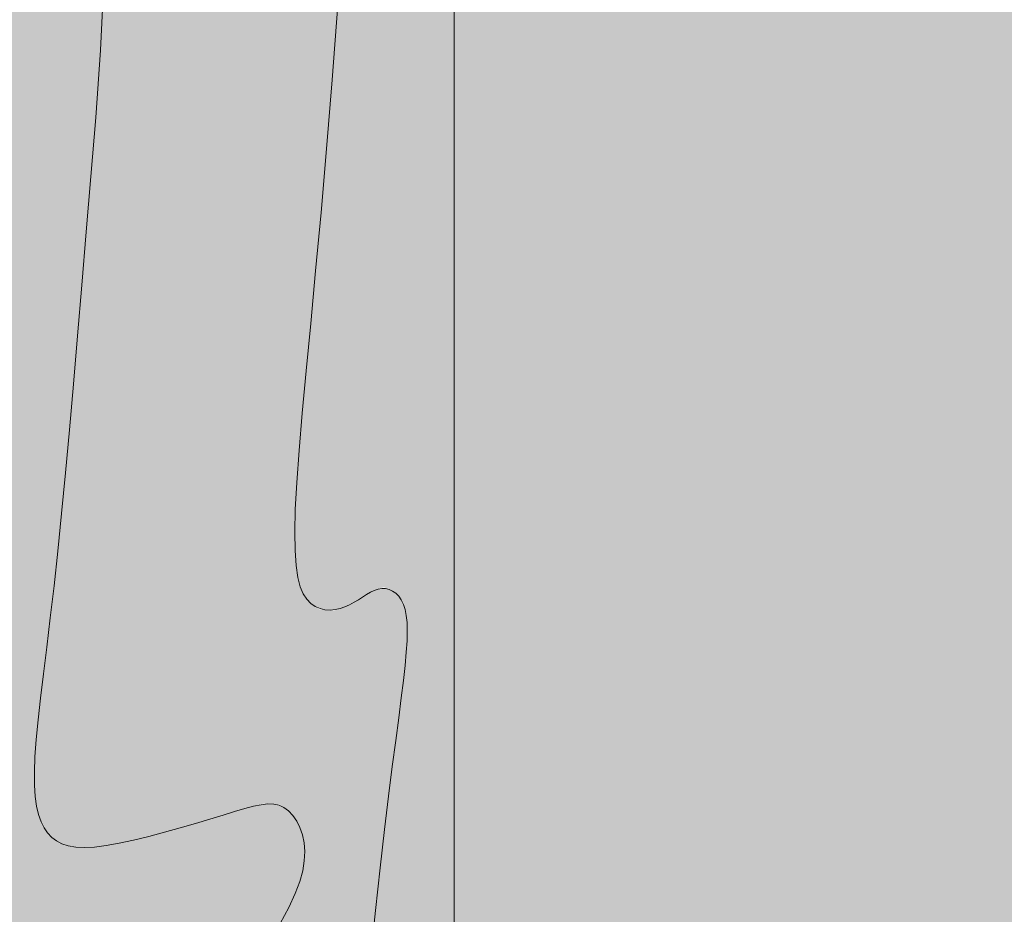
# Model space of a CAD drawing. Units: inches. Extents: x 3024 to 3952, y 1308 to 1863.
# Tile 17 of 29: x 3411.08 to 3430.42, y 1506.34 to 1523.92. Entities that reach past the tile are written whole.
import ezdxf

# ---------------------------------------------------------------- set-up
doc = ezdxf.new("R2010")
doc.units = ezdxf.units.IN
for name, color, linetype, lineweight in [('A-ANNO-DIMS', 2, 'Continuous', 18), ('A-FLOR-TILE-PATT', 7, 'Continuous', 13), ('A-FURN', 8, 'Continuous', 18), ('A-FURN-PATT', 9, 'Continuous', 13)]:
    doc.layers.add(name, color=color, linetype=linetype, lineweight=lineweight)
doc.layers.add('A-FLOR-PATT', color=254, linetype='Continuous', lineweight=13, true_color=0xfeeab9)
doc.styles.get("Standard").update_dxf_attribs({"font": 'arial.ttf'})
doc.dimstyles.get("Standard").update_dxf_attribs({"dimtxt": 0.18, "dimasz": 0.18, "dimexe": 0.18, "dimexo": 0.0625, "dimgap": 0.09, "dimtad": 0, "dimtih": 1, "dimtoh": 1, "dimdec": 4, "dimzin": 0, "dimdsep": 46, "dimtxsty": 'Standard', "dimcen": 0.09, "dimadec": 0, "dimazin": 0, "dimtfac": 1, "dimtdec": 4, "dimtofl": 0, "dimtmove": 0, "dimatfit": 3, "dimfxl": 1, "dimtolj": 1, "dimtzin": 0, "dimarcsym": 0})

# ---------------------------------------------------------------- blocks, each defined once
blk = doc.blocks.new('Table - Rectangular Woodgrain 60 x 30 in.')
blk.add_line((60, 0), (0, 0))
for points in [[(23.3616, -3.0508), (25.3333, -3.2), (27.1477, -3.3495), (28.8172, -3.4958), (30.3437, -3.636), (31.7291, -3.7667), (32.9756, -3.8849), (34.0849, -3.9875), (35.059, -4.0714), (35.9, -4.1334), (36.6114, -4.1711), (37.2041, -4.1854), (37.6906, -4.1779), (38.0833, -4.15), (38.3948, -4.1034), (38.6375, -4.0396), (38.8239, -3.9602), (38.9666, -3.8667), (39.0764, -3.7608), (39.1573, -3.6448), (39.2116, -3.521), (39.2416, -3.3917), (39.2498, -3.2593), (39.2385, -3.1261), (39.21, -2.9944), (39.1666, -2.8667), (39.111, -2.7447), (39.0468, -2.6281), (38.978, -2.5163), (38.9083, -2.4083), (38.8418, -2.3035), (38.7823, -2.201), (38.7337, -2.1001), (38.7, -2), (38.6844, -1.9003), (38.6875, -1.8021), (38.7094, -1.707), (38.75, -1.6167), (38.8094, -1.5326), (38.8875, -1.4563), (38.9844, -1.3893), (39.1, -1.3333), (39.2351, -1.2896), (39.3937, -1.2583), (39.5804, -1.2396), (39.8, -1.2333), (40.057, -1.2396), (40.3562, -1.2583), (40.7023, -1.2896), (41.1, -1.3333), (41.5547, -1.3895), (42.0755, -1.4573), (42.6721, -1.5361), (43.3542, -1.625), (44.1316, -1.7233), (45.014, -1.8302), (46.0114, -1.9449), (47.1333, -2.0667), (48.3862, -2.1947)], [(22.3952, -9.1759), (24.5531, -9.2844), (26.322, -9.4069), (27.8666, -9.5333), (29.3241, -9.6553), (30.7203, -9.7719), (32.0532, -9.8837), (33.3208, -9.9917), (34.5213, -10.0965), (35.6526, -10.199), (36.7128, -10.2999), (37.7, -10.4), (38.6129, -10.4996), (39.4531, -10.5969), (40.223, -10.6895), (40.925, -10.775), (41.5613, -10.8512), (42.1344, -10.9156), (42.6465, -10.966), (43.1, -11), (43.4976, -11.0158), (43.8437, -11.0136), (44.143, -10.9942), (44.4, -10.9583), (44.6195, -10.9069), (44.8062, -10.8406), (44.9648, -10.7603), (45.1, -10.6667), (45.2155, -10.5598), (45.3114, -10.4365), (45.3871, -10.2929), (45.4416, -10.125), (45.4743, -9.929), (45.4844, -9.7011), (45.4709, -9.4371), (45.4333, -9.1333), (45.3716, -8.7883), (45.2896, -8.4104), (45.1919, -8.0107), (45.0833, -7.6), (44.9685, -7.1893), (44.8521, -6.7896), (44.7388, -6.4117), (44.6333, -6.0667), (44.54, -5.7628), (44.4614, -5.4979), (44.4001, -5.2675), (44.3583, -5.0667), (44.3384, -4.8909), (44.3427, -4.7354), (44.3736, -4.5956), (44.4333, -4.4667), (44.5236, -4.3453), (44.6427, -4.2333), (44.7884, -4.1339), (44.9583, -4.05), (45.1501, -3.9849), (45.3614, -3.9417), (45.59, -3.9234), (45.8333, -3.9333), (46.0915, -3.9749), (46.3734, -4.0531), (46.6906, -4.1736), (47.0542, -4.3417), (47.4756, -4.5629)]]:
    blk.add_lwpolyline(points)
blk = doc.blocks.new('*D104')
at = {"layer": 'A-ANNO-DIMS', "color": 0, "lineweight": -2, "transparency": 16777216}
for p, q in [((3360.738, 1515.697), (3360.738, 1515.877)), ((3360.648, 1515.787), (3360.828, 1515.787)), ((3507.355, 1515.787), (3452.554, 1515.787))]:
    blk.add_line(p, q, dxfattribs=at)
at = {"layer": 'A-ANNO-DIMS', "color": 0, "transparency": 16777216}
blk.add_solid([(3452.554, 1515.817), (3452.554, 1515.757), (3452.374, 1515.787)], dxfattribs=at)
at = {"layer": 'Defpoints', "color": 0, "transparency": 16777216}
for p in [(3360.738, 1515.787), (3452.374, 1515.787)]:
    blk.add_point(p, dxfattribs=at)
at = {"layer": 'A-ANNO-DIMS', "color": 0, "transparency": 16777216, "insert": (3507.835, 1515.787), "char_height": 0.18, "attachment_point": 5}
blk.add_mtext('\\A1;R91.64', dxfattribs=at)
blk = doc.blocks.new('*D105')
at = {"layer": 'A-ANNO-DIMS', "color": 0, "lineweight": -2, "transparency": 16777216}
for p, q in [((3370.527, 1515.697), (3370.527, 1515.877)), ((3370.437, 1515.787), (3370.617, 1515.787)), ((3508.74, 1515.787), (3457.09, 1515.787))]:
    blk.add_line(p, q, dxfattribs=at)
at = {"layer": 'A-ANNO-DIMS', "color": 0, "transparency": 16777216}
blk.add_solid([(3457.09, 1515.817), (3457.09, 1515.757), (3456.91, 1515.787)], dxfattribs=at)
at = {"layer": 'Defpoints', "color": 0, "transparency": 16777216}
for p in [(3370.527, 1515.787), (3456.91, 1515.787)]:
    blk.add_point(p, dxfattribs=at)
at = {"layer": 'A-ANNO-DIMS', "color": 0, "transparency": 16777216, "insert": (3509.22, 1515.787), "char_height": 0.18, "attachment_point": 5}
blk.add_mtext('\\A1;R86.38', dxfattribs=at)

msp = doc.modelspace()

# ---------------------------------------------------------------- hatches: boundary and pattern name
at = {"layer": 'A-FLOR-PATT', "transparency": 33554528}
h = msp.add_hatch(color=256, dxfattribs=at)
h.dxf.hatch_style = 1
h.paths.add_polyline_path([(3460.764, 1688.6064), (3412.764, 1688.6064), (3412.764, 1694.6064), (3460.764, 1694.6064), (3460.764, 1778.6064), (3406.764, 1778.6064), (3406.764, 1759.9514), (3318.2981, 1759.9514), (3318.2981, 1658.6064), (3322.5356, 1658.6064), (3322.5356, 1652.6064), (3292.764, 1652.6064), (3292.764, 1778.6064), (3106.764, 1778.6064), (3106.764, 1628.6064), (3172.764, 1628.6064), (3172.764, 1532.6064), (3166.764, 1532.6064), (3166.764, 1628.6064), (3106.764, 1628.6064), (3106.764, 1356.8452), (3202.812, 1356.8452), (3202.812, 1354.2534), (3202.812, 1353.8388), (3202.812, 1351.1212), (3202.812, 1347.8452), (3277.764, 1347.8452), (3277.764, 1353.8452), (3277.764, 1356.8452), (3277.764, 1442.6064), (3460.764, 1442.6064)])
h.paths.add_polyline_path([(3216.238, 1527.2064), (3216.238, 1491.2064), (3214.663, 1491.2064), (3214.663, 1491.2409, -0.3966224), (3180.243, 1526.6064), (3163.0285, 1526.6064), (3163.0285, 1531.1064), (3161.716, 1531.1064), (3161.716, 1561.1064), (3163.0285, 1561.1064), (3163.0285, 1531.1064), (3163.0285, 1526.6064), (3180.243, 1526.6064, 0.3966224), (3214.663, 1491.2409), (3214.663, 1527.2064)], flags=16)
h.paths.add_polyline_path([(3227.364, 1649.8972), (3191.364, 1649.8972), (3191.364, 1651.4722), (3227.364, 1651.4722)], flags=16)
h.paths.add_polyline_path([(3323.1172, 1606.7362), (3323.8545, 1606.8514), (3323.8545, 1594.8241), (3323.1172, 1594.9393)], flags=16)
h.paths.add_polyline_path([(3324.2232, 1606.909), (3330.1216, 1607.8307), (3330.1216, 1614.1093), (3339.3495, 1614.1093), (3340.2711, 1620.0078), (3352.4136, 1620.0078), (3353.3353, 1614.1093), (3359.9941, 1614.1093), (3360.9157, 1620.0078), (3373.0582, 1620.0078), (3373.9799, 1614.1093), (3383.2077, 1614.1093), (3383.2077, 1607.8307), (3389.1062, 1606.909), (3389.1062, 1594.7665), (3383.2077, 1593.8449), (3383.2077, 1587.5663), (3373.9799, 1587.5663), (3373.0583, 1581.6678), (3360.9157, 1581.6678), (3359.9941, 1587.5663), (3353.3353, 1587.5663), (3352.4136, 1581.6678), (3340.2711, 1581.6678), (3339.3495, 1587.5663), (3330.1216, 1587.5663), (3330.1216, 1593.8449), (3324.2232, 1594.7665)], flags=16)
h.paths.add_polyline_path([(3236.1584, 1693.1064), (3236.1584, 1723.1064), (3237.4709, 1723.1064), (3237.4709, 1693.1064)], flags=16)
h.paths.add_polyline_path([(3373.2158, 1600.6847), (3373.7965, 1600.7303), (3374.3268, 1600.7874), (3374.8132, 1600.8531), (3375.2621, 1600.9247), (3375.6801, 1600.9991), (3376.0736, 1601.0735), (3376.6855, 1601.19), (3377.366, 1601.3023), (3378.0667, 1601.3814), (3378.8026, 1601.4123), (3379.5865, 1601.3839), (3380.4537, 1601.2948), (3381.301, 1601.1717), (3382.0317, 1601.0433), (3382.4398, 1600.9607), (3382.6252, 1600.9201), (3382.919, 1600.8507), (3382.9044, 1600.8531), (3382.842, 1600.8678), (3382.7541, 1600.8896), (3382.6252, 1600.9201), (3382.4398, 1600.9607), (3382.1868, 1601.0119), (3381.8738, 1601.0711), (3381.5125, 1601.1346), (3381.1149, 1601.1988), (3380.6928, 1601.2601), (3380.2581, 1601.3149), (3379.8226, 1601.3597), (3379.3984, 1601.3908), (3378.9944, 1601.4054), (3378.6092, 1601.4042), (3378.2384, 1601.3886), (3377.8777, 1601.36), (3377.5227, 1601.32), (3377.1691, 1601.2698), (3376.8127, 1601.211), (3376.4491, 1601.145), (3376.0736, 1601.0735), (3375.4177, 1600.9494), (3374.5542, 1600.8119), (3373.5044, 1600.6988)], flags=0)
h.paths.add_polyline_path([(3380.0253, 1596.7351), (3380.499, 1596.6659), (3380.9706, 1596.6119), (3381.4375, 1596.5791), (3381.8971, 1596.5736), (3382.5886, 1596.6167), (3382.7848, 1596.6692), (3382.1465, 1596.5706), (3381.236, 1596.5815), (3380.3199, 1596.6865)], flags=0)
h.paths.add_polyline_path([(3369.6414, 1603.9617), (3370.1589, 1604.0021), (3370.6218, 1604.0539), (3371.0335, 1604.1173), (3371.3978, 1604.1921), (3371.7181, 1604.2785), (3371.9984, 1604.3761), (3372.2441, 1604.483), (3372.4611, 1604.5972), (3372.655, 1604.7163), (3372.8317, 1604.8384), (3372.9968, 1604.9611), (3373.3703, 1605.2455), (3373.8426, 1605.5328), (3374.4624, 1605.7539), (3375.1058, 1605.8302), (3375.7221, 1605.8261), (3376.4109, 1605.76), (3377.1534, 1605.6376), (3377.8945, 1605.473), (3378.1382, 1605.409), (3377.7394, 1605.5074), (3377.3509, 1605.5937), (3376.9704, 1605.6677), (3376.5999, 1605.7288), (3376.2417, 1605.7762), (3375.8979, 1605.8092), (3375.5707, 1605.8271), (3375.2621, 1605.8291), (3374.9745, 1605.8146), (3374.7092, 1605.7832), (3374.4647, 1605.7359), (3374.239, 1605.6742), (3374.0298, 1605.5996), (3373.835, 1605.5134), (3373.6525, 1605.4171), (3373.4801, 1605.3123), (3373.3156, 1605.2002), (3373.1562, 1605.0825), (3372.7603, 1604.781), (3372.236, 1604.4588), (3371.5738, 1604.2283), (3370.8493, 1604.0794), (3369.9262, 1603.976)], flags=0)
h.paths.add_polyline_path([(3366.7533, 1606.5832), (3367.1713, 1606.5519), (3367.5378, 1606.5374), (3367.8568, 1606.5394), (3368.1325, 1606.5573), (3368.3694, 1606.5903), (3368.5717, 1606.6377), (3368.7438, 1606.6988), (3368.89, 1606.7728), (3369.0146, 1606.8591), (3369.121, 1606.9568), (3369.2094, 1607.0646), (3369.2792, 1607.181), (3369.3295, 1607.3046), (3369.3596, 1607.4339), (3369.3688, 1607.5676), (3369.3565, 1607.7042), (3369.3218, 1607.8422), (3369.2649, 1607.9804), (3369.1893, 1608.1187), (3369.0993, 1608.2569), (3368.9992, 1608.3952), (3368.8934, 1608.5334), (3368.7861, 1608.6717), (3368.6817, 1608.8099), (3368.4212, 1609.1804), (3368.2685, 1609.7106), (3368.4883, 1610.1814), (3369.0537, 1610.4604), (3369.6717, 1610.5097), (3370.2812, 1610.3612), (3370.4805, 1610.2968), (3370.1882, 1610.3839), (3369.9284, 1610.4472), (3369.6905, 1610.4842), (3369.4662, 1610.4933), (3369.2555, 1610.4765), (3369.0608, 1610.4367), (3368.884, 1610.3767), (3368.7274, 1610.2994), (3368.5931, 1610.2077), (3368.4833, 1610.1045), (3368.4002, 1609.9927), (3368.3451, 1609.8747), (3368.3166, 1609.7517), (3368.3127, 1609.6244), (3368.331, 1609.4935), (3368.3696, 1609.3597), (3368.4261, 1609.2237), (3368.4985, 1609.0863), (3368.5845, 1608.9482), (3368.6817, 1608.8099), (3368.7861, 1608.6717), (3368.8934, 1608.5334), (3368.9992, 1608.3952), (3369.0993, 1608.2569), (3369.3398, 1607.8876), (3369.3941, 1607.2896), (3368.9774, 1606.7817), (3368.3928, 1606.5742), (3367.7162, 1606.5303), (3367.0044, 1606.5585)], flags=0)
h.paths.add_polyline_path([(3362.1859, 1610.2589), (3362.5478, 1610.2845), (3362.8348, 1610.3275), (3363.0585, 1610.3863), (3363.2303, 1610.4595), (3363.3619, 1610.5457), (3363.463, 1610.6432), (3363.5376, 1610.7502), (3363.5876, 1610.8643), (3363.6153, 1610.9834), (3363.6229, 1611.1055), (3363.6125, 1611.2283), (3363.5861, 1611.3496), (3363.5462, 1611.4673), (3363.4949, 1611.5797), (3363.4358, 1611.6871), (3363.3723, 1611.7902), (3363.3081, 1611.8897), (3363.2468, 1611.9863), (3363.192, 1612.0808), (3363.0258, 1612.4261), (3363.3371, 1612.8672), (3363.9008, 1612.9782), (3364.4822, 1612.9641), (3365.1098, 1612.9074), (3365.328, 1612.8805), (3364.9615, 1612.9208), (3364.6426, 1612.9496), (3364.3668, 1612.9669), (3364.1299, 1612.9726), (3363.9276, 1612.9669), (3363.7555, 1612.9496), (3363.6093, 1612.9208), (3363.4848, 1612.8805), (3363.3782, 1612.8289), (3363.2889, 1612.7672), (3363.2169, 1612.6969), (3363.1622, 1612.6193), (3363.1247, 1612.5361), (3363.1046, 1612.4484), (3363.1017, 1612.358), (3363.1161, 1612.266), (3363.1472, 1612.1738), (3363.192, 1612.0808), (3363.2468, 1611.9863), (3363.3081, 1611.8897), (3363.3723, 1611.7902), (3363.4358, 1611.6871), (3363.6363, 1611.323), (3363.5979, 1610.7003), (3363.0863, 1610.3651), (3362.3983, 1610.2622)], flags=0)
h.paths.add_polyline_path([(3352.356, 1581.2991), (3352.2408, 1580.5618), (3340.4439, 1580.5618), (3340.3287, 1581.2991)], flags=16)
h.paths.add_polyline_path([(3340.4439, 1621.1137), (3352.2408, 1621.1137), (3352.356, 1620.3764), (3340.3287, 1620.3764)], flags=16)
h.paths.add_polyline_path([(3278.4282, 1504.7424), (3290.3831, 1504.7424), (3290.3831, 1502.7499), (3291.0473, 1502.7499), (3291.0473, 1494.7799), (3290.3831, 1494.7799), (3290.3831, 1494.1158), (3291.0473, 1494.1158), (3291.0473, 1486.1458), (3290.3831, 1486.1458), (3290.3831, 1484.1533), (3291.0473, 1484.1533), (3291.0473, 1483.4892, -0.0909091), (3291.0473, 1468.8776), (3291.0473, 1468.2135), (3290.3831, 1468.2135), (3290.3831, 1464.8926), (3278.4282, 1464.8926), (3278.4282, 1472.8626), (3277.764, 1473.5268), (3277.764, 1478.84), (3278.4282, 1479.5042)], flags=16)
h.paths.add_polyline_path([(3278.7603, 1504.4103), (3290.051, 1504.4103), (3290.051, 1465.2247), (3278.7603, 1465.2247)], flags=0)
h.paths.add_polyline_path([(3123.904, 1600.7821), (3117.9039, 1602.7821), (3117.9039, 1599.7821), (3119.4039, 1599.7821), (3119.4039, 1596.7821), (3118.4039, 1596.7821), (3118.4039, 1598.7821), (3117.9039, 1598.7821), (3117.9039, 1596.2821), (3109.9039, 1596.2821), (3109.9039, 1617.2821), (3117.9039, 1617.2821), (3117.9039, 1610.7821), (3123.9038, 1612.7821, -0.7025712), (3137.9039, 1606.7822, -0.7025621)], flags=16)
h.paths.add_polyline_path([(3123.9039, 1602.7822), (3123.9039, 1610.7822, -0.7345333), (3136.9039, 1606.7822, -0.7345297)], flags=0)
h.paths.add_polyline_path([(3177.972, 1689.6473), (3109.2405, 1689.6473), (3109.2405, 1741.1959), (3177.972, 1741.1959)], flags=16)
h.paths.add_polyline_path([(3373.0006, 1581.2991), (3372.8854, 1580.5618), (3361.0885, 1580.5618), (3360.9733, 1581.2991)], flags=16)
h.paths.add_polyline_path([(3361.0885, 1621.1137), (3372.8854, 1621.1137), (3373.0006, 1620.3764), (3360.9733, 1620.3764)], flags=16)
h.paths.add_polyline_path([(3116.9039, 1598.2821, -0.4142136), (3116.1539, 1597.2821), (3111.9039, 1597.2821, -0.4142136), (3110.9039, 1598.0321), (3110.9039, 1615.2821, -0.4142136), (3111.6539, 1616.2821), (3115.9039, 1616.2821, -0.4142136), (3116.9039, 1615.5321)], flags=0)
h.paths.add_polyline_path([(3121.6122, 1728.1369), (3121.6122, 1696.5205), (3110.2715, 1696.5205), (3110.2715, 1714.3906), (3121.6122, 1714.3906), (3121.6122, 1716.4526), (3110.2715, 1716.4526), (3110.2715, 1734.3228), (3123.3304, 1734.3228), (3123.3304, 1729.8552), (3134.6711, 1741.1959), (3134.6711, 1728.1369)], flags=0)
h.paths.add_polyline_path([(3389.4748, 1606.8514), (3390.2122, 1606.7362), (3390.2122, 1594.9393), (3389.4748, 1594.8241)], flags=16)
h.paths.add_polyline_path([(3257.6842, 1762.8281), (3259.6842, 1768.8281), (3256.6842, 1768.8281), (3256.6842, 1767.3281), (3253.6842, 1767.3281), (3253.6842, 1768.3281), (3255.6842, 1768.3281), (3255.6842, 1768.8281), (3253.1842, 1768.8281), (3253.1842, 1776.8281), (3274.1842, 1776.8281), (3274.1842, 1768.8281), (3267.6842, 1768.8281), (3269.6842, 1762.8282, -0.7025712), (3263.6843, 1748.8282, -0.7025621)], flags=16)
h.paths.add_polyline_path([(3259.6842, 1762.8281), (3267.6843, 1762.8281, -0.7345333), (3263.6842, 1749.8282, -0.7345297)], flags=0)
h.paths.add_polyline_path([(3411.264, 1715.6064), (3411.264, 1716.9189), (3441.264, 1716.9189), (3441.264, 1715.6064)], flags=16)
h.paths.add_polyline_path([(3178.3806, 1449.1876), (3178.3806, 1397.639), (3109.6491, 1397.639), (3109.6491, 1449.1876)], flags=16)
h.paths.add_polyline_path([(3397.1501, 1541.7146), (3419.6183, 1541.7146), (3419.6183, 1496.7783), (3397.1501, 1496.7783)], flags=16)
h.paths.add_polyline_path([(3254.1842, 1770.5781), (3254.1842, 1774.8281, -0.4142136), (3254.9342, 1775.8281), (3272.1842, 1775.8281, -0.4142136), (3273.1842, 1775.0781), (3273.1842, 1770.8281, -0.4142136), (3272.4342, 1769.8281), (3255.1842, 1769.8281, -0.4142136)], flags=0)
h.paths.add_polyline_path([(3403.672, 1500.7601), (3403.6016, 1500.3997), (3403.5328, 1500.0441), (3403.4662, 1499.6867), (3403.4027, 1499.3226), (3403.3464, 1498.9532), (3403.3025, 1498.5811), (3403.2759, 1498.2091), (3403.2714, 1497.8401), (3403.3064, 1497.2813), (3403.3491, 1497.1219), (3403.2689, 1497.6395), (3403.2778, 1498.3719), (3403.3635, 1499.0984), (3403.4889, 1499.8168), (3403.6016, 1500.3997), (3403.672, 1500.7601), (3403.744, 1501.1315), (3403.817, 1501.5205), (3403.891, 1501.9336), (3403.9656, 1502.3769), (3404.0404, 1502.8572), (3404.115, 1503.3786), (3404.2264, 1504.2311), (3404.2571, 1504.5223), (3404.1552, 1503.6598), (3404.0063, 1502.6193), (3403.8604, 1501.7518), (3403.744, 1501.1315)], flags=0)
h.paths.add_polyline_path([(3406.5868, 1505.0416), (3406.6121, 1504.5236), (3406.6492, 1504.0526), (3406.6956, 1503.624), (3406.7491, 1503.2333), (3406.8072, 1502.8759), (3406.8676, 1502.5473), (3406.9281, 1502.243), (3407.0268, 1501.7597), (3407.1416, 1501.1368), (3407.2087, 1500.3904), (3407.1804, 1499.6703), (3407.1078, 1498.9956), (3407.0074, 1498.3199), (3406.8809, 1497.6059), (3406.7403, 1496.9627), (3406.7418, 1496.9824), (3406.7491, 1497.0249), (3406.8229, 1497.3409), (3406.8364, 1497.4025), (3406.878, 1497.6078), (3406.9261, 1497.8614), (3406.9777, 1498.1526), (3407.0298, 1498.4712), (3407.0797, 1498.8068), (3407.1243, 1499.149), (3407.1607, 1499.4874), (3407.1859, 1499.8115), (3407.1978, 1500.1137), (3407.1969, 1500.3962), (3407.1841, 1500.6642), (3407.1609, 1500.9225), (3407.1284, 1501.1761), (3407.0876, 1501.43), (3407.0398, 1501.6891), (3406.9862, 1501.9585), (3406.8832, 1502.4628), (3406.7712, 1503.0713), (3406.6657, 1503.8424), (3406.5924, 1504.7735)], flags=0)
h.paths.add_polyline_path([(3409.2517, 1507.8962), (3409.2752, 1507.4282), (3409.3079, 1507.0076), (3409.3501, 1506.6314), (3409.4015, 1506.2969), (3409.4624, 1506.0009), (3409.5326, 1505.7406), (3409.6119, 1505.5128), (3409.6988, 1505.3131), (3409.7915, 1505.1368), (3409.8883, 1504.9792), (3409.9875, 1504.8356), (3410.0872, 1504.7015), (3410.1859, 1504.572), (3410.4508, 1504.2132), (3410.7205, 1503.6035), (3410.8059, 1502.8824), (3410.7619, 1502.0875), (3410.6122, 1501.2299), (3410.4402, 1500.6169), (3410.2538, 1500.0031), (3410.0536, 1499.3219), (3409.9909, 1499.0812), (3410.1761, 1499.7472), (3410.3596, 1500.3513), (3410.4512, 1500.6561), (3410.5312, 1500.9412), (3410.6013, 1501.226), (3410.6614, 1501.512), (3410.7111, 1501.7964), (3410.7496, 1502.0763), (3410.7764, 1502.3489), (3410.7909, 1502.6114), (3410.7926, 1502.8608), (3410.7808, 1503.0944), (3410.7553, 1503.31), (3410.7169, 1503.5087), (3410.6667, 1503.6921), (3410.6061, 1503.8621), (3410.5361, 1504.0203), (3410.4578, 1504.1686), (3410.3726, 1504.3088), (3410.2815, 1504.4424), (3410.1859, 1504.572), (3410.0872, 1504.7015), (3409.859, 1505.0083), (3409.5943, 1505.5117), (3409.4266, 1506.1336), (3409.324, 1506.8011), (3409.2586, 1507.6407)], flags=0)
h.paths.add_polyline_path([(3411.4914, 1510.5878), (3411.4432, 1510.1586), (3411.4054, 1509.775), (3411.38, 1509.4354), (3411.3681, 1509.1376), (3411.3698, 1508.8784), (3411.3843, 1508.6542), (3411.4112, 1508.4618), (3411.4497, 1508.2974), (3411.4994, 1508.1575), (3411.5595, 1508.0388), (3411.6296, 1507.9375), (3411.7097, 1507.851), (3411.802, 1507.7792), (3411.9096, 1507.7225), (3412.0353, 1507.6817), (3412.1821, 1507.6572), (3412.3528, 1507.6496), (3412.5505, 1507.6597), (3412.778, 1507.6879), (3413.0364, 1507.7341), (3413.3194, 1507.7955), (3413.6188, 1507.8687), (3413.9264, 1507.95), (3414.234, 1508.036), (3414.5333, 1508.1232), (3414.8163, 1508.208), (3415.0747, 1508.287), (3415.3023, 1508.3569), (3415.5007, 1508.4158), (3415.6733, 1508.4617), (3416.1158, 1508.5538), (3416.512, 1508.2591), (3416.716, 1507.6581), (3416.61, 1507.0003), (3416.3052, 1506.3411), (3415.8928, 1505.618), (3415.7339, 1505.3633), (3415.9914, 1505.791), (3416.201, 1506.1583), (3416.3666, 1506.4739), (3416.4925, 1506.7462), (3416.5828, 1506.9838), (3416.6413, 1507.1949), (3416.6725, 1507.3883), (3416.6799, 1507.5705), (3416.6662, 1507.7417), (3416.6339, 1507.9), (3416.5851, 1508.0436), (3416.5223, 1508.1709), (3416.4478, 1508.28), (3416.3639, 1508.3692), (3416.273, 1508.4368), (3416.1765, 1508.4815), (3416.0718, 1508.5047), (3415.9553, 1508.5079), (3415.8237, 1508.493), (3415.6733, 1508.4617), (3415.5007, 1508.4158), (3415.3327, 1508.3659), (3414.6495, 1508.157), (3414.0606, 1507.9855), (3413.4456, 1507.8229), (3412.8838, 1507.701), (3412.5505, 1507.6597), (3412.0748, 1507.6354), (3411.595, 1507.8883), (3411.398, 1508.4429), (3411.3624, 1508.9927), (3411.3854, 1509.5711), (3411.4578, 1510.3071)], flags=0)
h.paths.add_polyline_path([(3135.0797, 1449.1876), (3135.0797, 1436.1286), (3122.0208, 1436.1286), (3122.0208, 1404.5122), (3110.6801, 1404.5122), (3110.6801, 1422.3823), (3122.0208, 1422.3823), (3122.0208, 1424.4443), (3110.6801, 1424.4443), (3110.6801, 1442.3145), (3123.739, 1442.3145), (3123.739, 1437.8469)], flags=0)
h.paths.add_polyline_path([(3416.4944, 1514.2949), (3416.4837, 1513.8511), (3416.4893, 1513.4867), (3416.5102, 1513.1926), (3416.5451, 1512.9593), (3416.5929, 1512.7775), (3416.6524, 1512.6379), (3416.7224, 1512.531), (3416.8017, 1512.4488), (3416.8886, 1512.3882), (3416.9813, 1512.3476), (3417.0781, 1512.3251), (3417.1773, 1512.3189), (3417.277, 1512.3274), (3417.3757, 1512.3488), (3417.4713, 1512.3813), (3417.5627, 1512.4229), (3417.65, 1512.471), (3417.7338, 1512.5225), (3417.8146, 1512.5747), (3417.8931, 1512.6245), (3417.9699, 1512.6691), (3418.2968, 1512.8265), (3418.6505, 1512.4645), (3418.7037, 1511.9342), (3418.6693, 1511.3839), (3418.6076, 1510.8228), (3418.5777, 1510.5927), (3418.6197, 1510.9333), (3418.6525, 1511.2311), (3418.6759, 1511.4903), (3418.6899, 1511.7144), (3418.6946, 1511.9069), (3418.6899, 1512.0713), (3418.6759, 1512.2112), (3418.6525, 1512.33), (3418.6197, 1512.4311), (3418.5778, 1512.5177), (3418.5276, 1512.5903), (3418.4705, 1512.6488), (3418.4075, 1512.6933), (3418.3399, 1512.7237), (3418.2686, 1512.7401), (3418.1951, 1512.7424), (3418.1204, 1512.7307), (3418.0455, 1512.7055), (3417.9792, 1512.6736), (3417.65, 1512.471), (3417.5627, 1512.4229), (3417.4713, 1512.3813), (3417.3757, 1512.3488), (3417.277, 1512.3274), (3416.878, 1512.2936), (3416.5757, 1512.7549), (3416.492, 1513.3145), (3416.4808, 1514.0384)], flags=0)
h.paths.add_polyline_path([(3392.8223, 1481.9454), (3396.7707, 1481.9454), (3396.7707, 1480.9201), (3428.3585, 1480.9201), (3428.3585, 1481.9454), (3432.3069, 1481.9454), (3432.3069, 1464.8354, -0.266667), (3392.8223, 1464.8354)], flags=16)
h.paths.add_polyline_path([(3431.203, 1547.5428), (3450.8613, 1547.5428, -0.1904762), (3450.8614, 1484.031), (3431.203, 1484.031), (3431.203, 1488.5675), (3432.3809, 1488.5675), (3432.3809, 1543.0062), (3431.203, 1543.0062)], flags=16)
h.paths.add_polyline_path([(3451.9233, 1524.86, -0.0496282), (3451.9233, 1506.7138), (3446.7921, 1506.7138), (3446.7921, 1524.86)], flags=0)
h.paths.add_polyline_path([(3460.764, 1436.6064), (3277.764, 1436.6064), (3277.764, 1356.8452), (3277.764, 1353.8452), (3460.764, 1353.8452)], flags=17)
h.paths.add_polyline_path([(3121.3033, 1577.378), (3153.693, 1577.378), (3153.693, 1586.6752), (3121.3033, 1586.6752)], flags=24)
h.paths.add_polyline_path([(3164.1457, 1464.1276), (3210.4801, 1464.1276), (3210.4801, 1473.4247), (3164.1457, 1473.4247)], flags=24)
h.paths.add_polyline_path([(3343.1909, 1505.8863), (3373.7236, 1505.8863), (3373.7236, 1515.1773), (3343.1909, 1515.1773)], flags=24)
h.paths.add_polyline_path([(3337.6353, 1564.2926), (3370.0189, 1564.2926), (3370.0189, 1573.5836), (3337.6353, 1573.5836)], flags=24)
h.paths.add_polyline_path([(3419.204, 1753.8578), (3453.3997, 1753.8578), (3453.3997, 1762.9956), (3419.204, 1762.9956)], flags=24)
h.paths.add_polyline_path([(3341.2523, 1701.0246), (3381.0761, 1701.0246), (3381.0761, 1710.3156), (3341.2523, 1710.3156)], flags=24)
h.paths.add_polyline_path([(3245.8895, 1726.2997), (3278.2793, 1726.2997), (3278.2793, 1735.5968), (3245.8895, 1735.5968)], flags=24)
h.paths.add_polyline_path([(3128.8045, 1668.6736), (3175.1389, 1668.6736), (3175.1389, 1677.9707), (3128.8045, 1677.9707)], flags=24)
h.paths.add_polyline_path([(3345.9997, 1396.0062), (3389.09, 1396.0062), (3389.09, 1405.3033), (3345.9997, 1405.3033)], flags=24)
at = {"layer": 'A-FLOR-TILE-PATT', "transparency": 33554569}
h = msp.add_hatch(dxfattribs=at)
h.set_pattern_fill('ANGLE', color=256, scale=2)
h.set_pattern_definition([(0, (0, 0), (0, 13.97), [10.16, -3.81]), (90, (0, 0), (-13.97, 9e-16), [10.16, -3.81])])
h.paths.add_polyline_path([(3292.764, 1778.6064), (3232.764, 1778.6064), (3232.764, 1694.6064), (3236.1584, 1694.6064), (3236.1584, 1723.1064), (3237.4709, 1723.1064), (3237.4709, 1723.0777, -0.3870039), (3266.1209, 1694.6064), (3292.764, 1694.6064)])
h.paths.add_polyline_path([(3263.6843, 1748.8282, -0.7025621), (3257.6842, 1762.8281), (3259.6842, 1768.8281), (3256.6842, 1768.8281), (3256.6842, 1767.3281), (3253.6842, 1767.3281), (3253.6842, 1768.3281), (3255.6842, 1768.3281), (3255.6842, 1768.8281), (3253.1842, 1768.8281), (3253.1842, 1776.8281), (3274.1842, 1776.8281), (3274.1842, 1768.8281), (3267.6842, 1768.8281), (3269.6842, 1762.8282, -0.7025712)], flags=16)
h.paths.add_polyline_path([(3263.6842, 1749.8282, -0.7345297), (3259.6842, 1762.8281), (3267.6843, 1762.8281, -0.7345333)], flags=0)
h.paths.add_polyline_path([(3255.1842, 1769.8281, -0.4142136), (3254.1842, 1770.5781), (3254.1842, 1774.8281, -0.4142136), (3254.9342, 1775.8281), (3272.1842, 1775.8281, -0.4142136), (3273.1842, 1775.0781), (3273.1842, 1770.8281, -0.4142136), (3272.4342, 1769.8281)], flags=0)
h.paths.add_polyline_path([(3460.764, 1436.6064), (3277.764, 1436.6064), (3277.764, 1356.8452), (3277.764, 1353.8452), (3460.764, 1353.8452)])
h.paths.add_polyline_path([(3166.764, 1628.6064), (3106.764, 1628.6064), (3106.764, 1532.6064), (3133.066, 1532.6064, -0.3870039), (3161.716, 1561.0777), (3161.716, 1561.1064), (3163.0285, 1561.1064), (3163.0285, 1532.6064), (3166.764, 1532.6064)])
h.paths.add_polyline_path([(3123.904, 1600.7821), (3117.9039, 1602.7821), (3117.9039, 1599.7821), (3119.4039, 1599.7821), (3119.4039, 1596.7821), (3118.4039, 1596.7821), (3118.4039, 1598.7821), (3117.9039, 1598.7821), (3117.9039, 1596.2821), (3109.9039, 1596.2821), (3109.9039, 1617.2821), (3117.9039, 1617.2821), (3117.9039, 1610.7821), (3123.9038, 1612.7821, -0.7025712), (3137.9039, 1606.7822, -0.7025621)], flags=16)
h.paths.add_polyline_path([(3123.9039, 1602.7822), (3123.9039, 1610.7822, -0.7345333), (3136.9039, 1606.7822, -0.7345297)], flags=0)
h.paths.add_polyline_path([(3116.1539, 1597.2821), (3111.9039, 1597.2821, -0.4142136), (3110.9039, 1598.0321), (3110.9039, 1615.2821, -0.4142136), (3111.6539, 1616.2821), (3115.9039, 1616.2821, -0.4142136), (3116.9039, 1615.5321), (3116.9039, 1598.2821, -0.4142136)], flags=0)
h.paths.add_polyline_path([(3245.8895, 1726.2997), (3278.2793, 1726.2997), (3278.2793, 1735.5968), (3245.8895, 1735.5968)], flags=24)
h.paths.add_polyline_path([(3345.9997, 1396.0062), (3389.09, 1396.0062), (3389.09, 1405.3033), (3345.9997, 1405.3033)], flags=24)
h.paths.add_polyline_path([(3121.3033, 1577.378), (3153.693, 1577.378), (3153.693, 1586.6752), (3121.3033, 1586.6752)], flags=24)
at = {"layer": 'A-FURN-PATT', "transparency": 33554600}
h = msp.add_hatch(color=256, dxfattribs=at)
h.dxf.hatch_style = 1
h.paths.add_polyline_path([(3417.3334, 1524.2182), (3417.4417, 1525.8535), (3417.5429, 1527.6959), (3417.6336, 1529.794), (3417.7102, 1532.1964), (3417.7693, 1534.9516), (3417.8074, 1538.1081), (3417.8209, 1541.7146), (3412.7281, 1541.7146), (3412.8136, 1536.7897), (3412.8505, 1532.7734), (3412.8466, 1529.5424), (3412.8092, 1526.9731), (3412.7461, 1524.942), (3412.6649, 1523.3259), (3412.5731, 1522.0011), (3412.4784, 1520.8443), (3412.3871, 1519.7527), (3412.2998, 1518.707), (3412.216, 1517.7088), (3412.1351, 1516.7594), (3412.0566, 1515.8603), (3411.9799, 1515.013), (3411.9043, 1514.219), (3411.8293, 1513.4797), (3411.7548, 1512.7959), (3411.6819, 1512.1667), (3411.6125, 1511.5901), (3411.5485, 1511.0643), (3411.4914, 1510.5878), (3411.4432, 1510.1586), (3411.4054, 1509.775), (3411.38, 1509.4354), (3411.3681, 1509.1376), (3411.3698, 1508.8784), (3411.3843, 1508.6542), (3411.4112, 1508.4618), (3411.4497, 1508.2974), (3411.4994, 1508.1575), (3411.5595, 1508.0388), (3411.6296, 1507.9375), (3411.7097, 1507.851), (3411.802, 1507.7792), (3411.9096, 1507.7225), (3412.0353, 1507.6817), (3412.1821, 1507.6572), (3412.3528, 1507.6496), (3412.5505, 1507.6597), (3412.778, 1507.6879), (3413.0364, 1507.7341), (3413.3194, 1507.7955), (3413.6188, 1507.8687), (3413.9264, 1507.95), (3414.234, 1508.036), (3414.5333, 1508.1232), (3414.8163, 1508.208), (3415.0747, 1508.287), (3415.4508, 1508.4025), (3415.8572, 1508.5106), (3416.186, 1508.5015), (3416.4107, 1508.3344), (3416.5614, 1508.1136), (3416.6596, 1507.8241), (3416.6872, 1507.4795), (3416.6413, 1507.1949), (3416.5828, 1506.9838), (3416.4925, 1506.7462), (3416.3666, 1506.4739), (3416.201, 1506.1583), (3415.9914, 1505.791), (3415.7339, 1505.3633), (3415.4242, 1504.8669), (3415.0615, 1504.292), (3414.6566, 1503.6241), (3414.2236, 1502.8473), (3413.7766, 1501.946), (3413.3295, 1500.9042), (3412.8966, 1499.7062), (3412.4917, 1498.3362), (3412.1289, 1496.7783), (3417.2217, 1496.7783), (3417.334, 1498.1918), (3417.4456, 1499.5619), (3417.5561, 1500.8806), (3417.6648, 1502.1395), (3417.7712, 1503.3306), (3417.8747, 1504.4456), (3417.9746, 1505.4763), (3418.0705, 1506.4147), (3418.1617, 1507.2549), (3418.2476, 1508.0019), (3418.3277, 1508.6628), (3418.4013, 1509.245), (3418.4679, 1509.7559), (3418.5269, 1510.2027), (3418.5777, 1510.5927), (3418.6197, 1510.9333), (3418.6525, 1511.2311), (3418.6759, 1511.4903), (3418.6899, 1511.7144), (3418.6946, 1511.9069), (3418.6899, 1512.0713), (3418.6759, 1512.2112), (3418.6525, 1512.33), (3418.6197, 1512.4311), (3418.5778, 1512.5177), (3418.5276, 1512.5903), (3418.4705, 1512.6488), (3418.4075, 1512.6933), (3418.3399, 1512.7237), (3418.2686, 1512.7401), (3418.1951, 1512.7424), (3418.1204, 1512.7307), (3418.0455, 1512.7055), (3417.9699, 1512.6691), (3417.8931, 1512.6245), (3417.8146, 1512.5747), (3417.5633, 1512.4125), (3417.2709, 1512.3131), (3416.9695, 1512.3318), (3416.7549, 1512.4815), (3416.6143, 1512.696), (3416.5451, 1512.9593), (3416.5102, 1513.1926), (3416.4893, 1513.4867), (3416.4837, 1513.8511), (3416.4944, 1514.2949), (3416.5226, 1514.8277), (3416.5691, 1515.4576), (3416.6319, 1516.1871), (3416.7088, 1517.0179), (3416.7973, 1517.9515), (3416.8952, 1518.9891), (3417.0002, 1520.1323), (3417.1097, 1521.3827), (3417.2217, 1522.7416)])
h.paths.add_polyline_path([(3419.6183, 1541.7146), (3417.8209, 1541.7146), (3417.8074, 1538.1081), (3417.7693, 1534.9516), (3417.7102, 1532.1964), (3417.6336, 1529.794), (3417.5429, 1527.6959), (3417.4417, 1525.8535), (3417.3334, 1524.2182), (3417.2217, 1522.7416), (3417.1097, 1521.3827), (3417.0002, 1520.1323), (3416.8952, 1518.9891), (3416.7973, 1517.9515), (3416.7088, 1517.0179), (3416.6319, 1516.1871), (3416.5691, 1515.4576), (3416.5226, 1514.8277), (3416.4944, 1514.2949), (3416.4837, 1513.8511), (3416.4893, 1513.4867), (3416.5102, 1513.1926), (3416.5451, 1512.9593), (3416.5929, 1512.7775), (3416.6524, 1512.6379), (3416.7224, 1512.531), (3416.8017, 1512.4488), (3416.8886, 1512.3882), (3416.9813, 1512.3476), (3417.0781, 1512.3251), (3417.1773, 1512.3189), (3417.277, 1512.3274), (3417.3757, 1512.3488), (3417.4713, 1512.3813), (3417.5627, 1512.4229), (3417.65, 1512.471), (3417.7338, 1512.5225), (3417.9865, 1512.6856), (3418.237, 1512.7699), (3418.4785, 1512.6613), (3418.6304, 1512.4416), (3418.6876, 1512.1519), (3418.6969, 1511.8267), (3418.6759, 1511.4903), (3418.6525, 1511.2311), (3418.6197, 1510.9333), (3418.5777, 1510.5927), (3418.5269, 1510.2027), (3418.4679, 1509.7559), (3418.4013, 1509.245), (3418.3277, 1508.6628), (3418.2476, 1508.0019), (3418.1617, 1507.2549), (3418.0705, 1506.4147), (3417.9746, 1505.4763), (3417.8747, 1504.4456), (3417.7712, 1503.3306), (3417.6648, 1502.1395), (3417.5561, 1500.8806), (3417.4456, 1499.5619), (3417.334, 1498.1918), (3417.2217, 1496.7783), (3419.6183, 1496.7783)])
h.paths.add_polyline_path([(3412.5731, 1522.0011), (3412.6649, 1523.3259), (3412.7461, 1524.942), (3412.8092, 1526.9731), (3412.8466, 1529.5424), (3412.8505, 1532.7734), (3412.8136, 1536.7897), (3412.7281, 1541.7146), (3410.0319, 1541.7146), (3409.9329, 1537.8316), (3409.8579, 1534.5089), (3409.8028, 1531.6816), (3409.7635, 1529.2854), (3409.7359, 1527.2554), (3409.7159, 1525.5271), (3409.6994, 1524.0356), (3409.6824, 1522.7166), (3409.6614, 1521.5137), (3409.6364, 1520.405), (3409.6078, 1519.3771), (3409.5763, 1518.4164), (3409.5425, 1517.5096), (3409.5069, 1516.6432), (3409.4701, 1515.8036), (3409.4327, 1514.9775), (3409.3955, 1514.1549), (3409.3594, 1513.3392), (3409.3256, 1512.5376), (3409.2955, 1511.7571), (3409.2699, 1511.0046), (3409.2501, 1510.2873), (3409.2375, 1509.6121), (3409.233, 1508.986), (3409.2377, 1508.4145), (3409.2517, 1507.8962), (3409.2752, 1507.4282), (3409.3079, 1507.0076), (3409.3501, 1506.6314), (3409.4015, 1506.2969), (3409.4624, 1506.0009), (3409.5326, 1505.7406), (3409.6119, 1505.5128), (3409.6988, 1505.3131), (3409.7915, 1505.1368), (3409.8883, 1504.9792), (3409.9875, 1504.8356), (3410.0872, 1504.7015), (3410.3178, 1504.3987), (3410.5042, 1504.0923), (3410.643, 1503.7787), (3410.7431, 1503.4127), (3410.7808, 1503.0944), (3410.7926, 1502.8608), (3410.7909, 1502.6114), (3410.7764, 1502.3489), (3410.7496, 1502.0763), (3410.7111, 1501.7964), (3410.6614, 1501.512), (3410.6013, 1501.226), (3410.5312, 1500.9412), (3410.4512, 1500.6561), (3410.3596, 1500.3513), (3410.2538, 1500.0031), (3410.1317, 1499.5877), (3409.9909, 1499.0812), (3409.8291, 1498.4601), (3409.6438, 1497.7003), (3409.4327, 1496.7783), (3412.1289, 1496.7783), (3412.4917, 1498.3362), (3412.8966, 1499.7062), (3413.3295, 1500.9042), (3413.7766, 1501.946), (3414.2236, 1502.8473), (3414.6566, 1503.6241), (3415.0615, 1504.292), (3415.4242, 1504.8669), (3415.7339, 1505.3633), (3415.9914, 1505.791), (3416.201, 1506.1583), (3416.3666, 1506.4739), (3416.4925, 1506.7462), (3416.5828, 1506.9838), (3416.6413, 1507.1949), (3416.6725, 1507.3883), (3416.6799, 1507.5705), (3416.6662, 1507.7417), (3416.6339, 1507.9), (3416.5851, 1508.0436), (3416.5223, 1508.1709), (3416.4478, 1508.28), (3416.3639, 1508.3692), (3416.273, 1508.4368), (3416.1765, 1508.4815), (3416.0718, 1508.5047), (3415.9553, 1508.5079), (3415.8237, 1508.493), (3415.6733, 1508.4617), (3415.5007, 1508.4158), (3415.3023, 1508.3569), (3414.8599, 1508.2211), (3414.5333, 1508.1232), (3414.234, 1508.036), (3413.9264, 1507.95), (3413.6188, 1507.8687), (3413.3194, 1507.7955), (3412.8838, 1507.701), (3412.4382, 1507.6458), (3412.0995, 1507.6608), (3411.8501, 1507.7418), (3411.666, 1507.885), (3411.5226, 1508.092), (3411.4241, 1508.3695), (3411.3843, 1508.6542), (3411.3698, 1508.8784), (3411.3681, 1509.1376), (3411.38, 1509.4354), (3411.4054, 1509.775), (3411.4432, 1510.1586), (3411.4914, 1510.5878), (3411.5485, 1511.0643), (3411.6125, 1511.5901), (3411.6819, 1512.1667), (3411.7548, 1512.7959), (3411.8293, 1513.4797), (3411.9043, 1514.219), (3411.9799, 1515.013), (3412.0566, 1515.8603), (3412.1351, 1516.7594), (3412.216, 1517.7088), (3412.2998, 1518.707), (3412.3871, 1519.7527), (3412.4784, 1520.8443)])
h.paths.add_polyline_path([(3409.6614, 1521.5137), (3409.6824, 1522.7166), (3409.6994, 1524.0356), (3409.7159, 1525.5271), (3409.7359, 1527.2554), (3409.7635, 1529.2854), (3409.8028, 1531.6816), (3409.8579, 1534.5089), (3409.9329, 1537.8316), (3410.0319, 1541.7146), (3406.1374, 1541.7146), (3406.3416, 1537.8771), (3406.5076, 1534.4792), (3406.639, 1531.4763), (3406.7397, 1528.8235), (3406.8135, 1526.4762), (3406.8641, 1524.3896), (3406.8955, 1522.5188), (3406.9113, 1520.8193), (3406.915, 1519.2519), (3406.9086, 1517.8009), (3406.8933, 1516.4564), (3406.8708, 1515.2084), (3406.8423, 1514.0471), (3406.8095, 1512.9624), (3406.7738, 1511.9444), (3406.7366, 1510.9832), (3406.6994, 1510.0706), (3406.664, 1509.2052), (3406.6321, 1508.3879), (3406.6055, 1507.6192), (3406.5859, 1506.8996), (3406.5751, 1506.2298), (3406.5748, 1505.6103), (3406.5868, 1505.0416), (3406.6121, 1504.5236), (3406.6492, 1504.0526), (3406.6956, 1503.624), (3406.7491, 1503.2333), (3406.8072, 1502.8759), (3406.8676, 1502.5473), (3406.9281, 1502.243), (3407.0268, 1501.7597), (3407.1147, 1501.2828), (3407.1609, 1500.9225), (3407.1841, 1500.6642), (3407.1969, 1500.3962), (3407.1978, 1500.1137), (3407.1859, 1499.8115), (3407.1607, 1499.4874), (3407.1243, 1499.149), (3407.0797, 1498.8068), (3407.0298, 1498.4712), (3406.9777, 1498.1526), (3406.9261, 1497.8614), (3406.8567, 1497.4956), (3406.7944, 1497.2102), (3406.7609, 1497.0755), (3406.7491, 1497.0249), (3406.7418, 1496.9824), (3406.7381, 1496.9355), (3406.7367, 1496.8717), (3406.7366, 1496.7783), (3409.4327, 1496.7783), (3409.6438, 1497.7003), (3409.8291, 1498.4601), (3409.9909, 1499.0812), (3410.1317, 1499.5877), (3410.2538, 1500.0031), (3410.3596, 1500.3513), (3410.4512, 1500.6561), (3410.5312, 1500.9412), (3410.6013, 1501.226), (3410.6614, 1501.512), (3410.7111, 1501.7964), (3410.7496, 1502.0763), (3410.7764, 1502.3489), (3410.7909, 1502.6114), (3410.7926, 1502.8608), (3410.7808, 1503.0944), (3410.7553, 1503.31), (3410.7169, 1503.5087), (3410.6667, 1503.6921), (3410.6061, 1503.8621), (3410.5361, 1504.0203), (3410.4578, 1504.1686), (3410.3726, 1504.3088), (3410.2815, 1504.4424), (3410.1859, 1504.572), (3410.0109, 1504.8017), (3409.8298, 1505.064), (3409.6475, 1505.4106), (3409.5326, 1505.7406), (3409.4624, 1506.0009), (3409.4015, 1506.2969), (3409.3501, 1506.6314), (3409.3079, 1507.0076), (3409.2752, 1507.4282), (3409.2517, 1507.8962), (3409.2377, 1508.4145), (3409.233, 1508.986), (3409.2375, 1509.6121), (3409.2501, 1510.2873), (3409.2699, 1511.0046), (3409.2955, 1511.7571), (3409.3256, 1512.5376), (3409.3594, 1513.3392), (3409.3955, 1514.1549), (3409.4327, 1514.9775), (3409.4701, 1515.8036), (3409.5069, 1516.6432), (3409.5425, 1517.5096), (3409.5763, 1518.4164), (3409.6078, 1519.3771), (3409.6364, 1520.405)])
h.paths.add_polyline_path([(3406.9113, 1520.8193), (3406.8955, 1522.5188), (3406.8641, 1524.3896), (3406.8135, 1526.4762), (3406.7397, 1528.8235), (3406.639, 1531.4763), (3406.5076, 1534.4792), (3406.3416, 1537.8771), (3406.1374, 1541.7146), (3402.8421, 1541.7146), (3402.9543, 1535.7158), (3403.0659, 1530.9229), (3403.1765, 1527.1726), (3403.2852, 1524.3018), (3403.3916, 1522.1472), (3403.4951, 1520.5454), (3403.595, 1519.3334), (3403.6909, 1518.3478), (3403.7822, 1517.4515), (3403.8687, 1516.6123), (3403.9507, 1515.8241), (3404.0279, 1515.0805), (3404.1004, 1514.3756), (3404.1683, 1513.7032), (3404.2315, 1513.0571), (3404.29, 1512.4311), (3404.3436, 1511.8197), (3404.3914, 1511.2188), (3404.4322, 1510.6249), (3404.4648, 1510.0345), (3404.4879, 1509.4441), (3404.5007, 1508.8503), (3404.5017, 1508.2494), (3404.4897, 1507.6379), (3404.4643, 1507.0142), (3404.4265, 1506.3837), (3404.3783, 1505.7534), (3404.3212, 1505.1306), (3404.2571, 1504.5223), (3404.1879, 1503.936), (3404.115, 1503.3786), (3404.0404, 1502.8572), (3403.9656, 1502.3769), (3403.891, 1501.9336), (3403.817, 1501.5205), (3403.744, 1501.1315), (3403.672, 1500.7601), (3403.6016, 1500.3997), (3403.5328, 1500.0441), (3403.4662, 1499.6867), (3403.4027, 1499.3226), (3403.3464, 1498.9532), (3403.3025, 1498.5811), (3403.2759, 1498.2091), (3403.2714, 1497.8401), (3403.2941, 1497.4768), (3403.3491, 1497.1219), (3403.4412, 1496.7783), (3406.7346, 1496.7783), (3406.7393, 1496.9886), (3406.7787, 1497.147), (3406.8034, 1497.2517), (3406.8364, 1497.4025), (3406.878, 1497.6078), (3406.9261, 1497.8614), (3406.9777, 1498.1526), (3407.0298, 1498.4712), (3407.0797, 1498.8068), (3407.1243, 1499.149), (3407.1607, 1499.4874), (3407.1859, 1499.8115), (3407.1978, 1500.1137), (3407.1969, 1500.3962), (3407.1841, 1500.6642), (3407.1609, 1500.9225), (3407.1284, 1501.1761), (3407.0876, 1501.43), (3407.0398, 1501.6891), (3406.9862, 1501.9585), (3406.8832, 1502.4628), (3406.8072, 1502.8759), (3406.7491, 1503.2333), (3406.6956, 1503.624), (3406.6492, 1504.0526), (3406.6121, 1504.5236), (3406.5868, 1505.0416), (3406.5748, 1505.6103), (3406.5751, 1506.2298), (3406.5859, 1506.8996), (3406.6055, 1507.6192), (3406.6321, 1508.3879), (3406.664, 1509.2052), (3406.6994, 1510.0706), (3406.7366, 1510.9832), (3406.7738, 1511.9444), (3406.8095, 1512.9624), (3406.8423, 1514.0471), (3406.8708, 1515.2084), (3406.8933, 1516.4564), (3406.9086, 1517.8009), (3406.915, 1519.2519)])
h.paths.add_polyline_path([(3403.7822, 1517.4515), (3403.6909, 1518.3478), (3403.595, 1519.3334), (3403.4951, 1520.5454), (3403.3916, 1522.1472), (3403.2852, 1524.3018), (3403.1765, 1527.1726), (3403.0659, 1530.9229), (3402.9543, 1535.7158), (3402.8421, 1541.7146), (3400.7451, 1541.7146), (3400.8571, 1535.2472), (3400.9674, 1529.9544), (3401.0741, 1525.6837), (3401.1757, 1522.2828), (3401.2702, 1519.5992), (3401.3559, 1517.4806), (3401.4311, 1515.7745), (3401.494, 1514.3284), (3401.5433, 1513.0143), (3401.5798, 1511.8008), (3401.6046, 1510.6809), (3401.6188, 1509.6476), (3401.6237, 1508.6939), (3401.6203, 1507.8127), (3401.61, 1506.9971), (3401.5938, 1506.2399), (3401.5729, 1505.5342), (3401.5474, 1504.8723), (3401.518, 1504.2464), (3401.4846, 1503.6491), (3401.4478, 1503.0725), (3401.4078, 1502.509), (3401.3648, 1501.9509), (3401.3192, 1501.3905), (3401.2716, 1500.8219), (3401.2236, 1500.246), (3401.1775, 1499.6652), (3401.1351, 1499.0821), (3401.0986, 1498.4993), (3401.0699, 1497.9194), (3401.0513, 1497.3449), (3401.0446, 1496.7783), (3403.4412, 1496.7783), (3403.3491, 1497.1219), (3403.2941, 1497.4768), (3403.2714, 1497.8401), (3403.2759, 1498.2091), (3403.3025, 1498.5811), (3403.3464, 1498.9532), (3403.4027, 1499.3226), (3403.4662, 1499.6867), (3403.5328, 1500.0441), (3403.6016, 1500.3997), (3403.672, 1500.7601), (3403.744, 1501.1315), (3403.817, 1501.5205), (3403.891, 1501.9336), (3403.9656, 1502.3769), (3404.0404, 1502.8572), (3404.115, 1503.3786), (3404.1879, 1503.936), (3404.2571, 1504.5223), (3404.3212, 1505.1306), (3404.3783, 1505.7534), (3404.4265, 1506.3837), (3404.4643, 1507.0142), (3404.4897, 1507.6379), (3404.5017, 1508.2494), (3404.5007, 1508.8503), (3404.4879, 1509.4441), (3404.4648, 1510.0345), (3404.4322, 1510.6249), (3404.3914, 1511.2188), (3404.3436, 1511.8197), (3404.29, 1512.4311), (3404.2315, 1513.0571), (3404.1683, 1513.7032), (3404.1004, 1514.3756), (3404.0279, 1515.0805), (3403.9507, 1515.8241), (3403.8687, 1516.6123)])
h.paths.add_polyline_path([(3401.3559, 1517.4806), (3401.2702, 1519.5992), (3401.1757, 1522.2828), (3401.0741, 1525.6837), (3400.9674, 1529.9544), (3400.8571, 1535.2472), (3400.7451, 1541.7146), (3398.0489, 1541.7146), (3398.1477, 1537.4556), (3398.2213, 1533.8882), (3398.2727, 1530.9247), (3398.3047, 1528.4771), (3398.3204, 1526.4579), (3398.3227, 1524.7793), (3398.3144, 1523.3534), (3398.2985, 1522.0924), (3398.2775, 1520.9226), (3398.2525, 1519.825), (3398.2239, 1518.7946), (3398.1924, 1517.8266), (3398.1586, 1516.9159), (3398.1229, 1516.0576), (3398.0862, 1515.2468), (3398.0489, 1514.4783), (3398.0117, 1513.7461), (3397.9759, 1513.0393), (3397.9431, 1512.346), (3397.9147, 1511.6541), (3397.8921, 1510.9518), (3397.8768, 1510.2269), (3397.8703, 1509.4674), (3397.8741, 1508.6615), (3397.8906, 1507.7925), (3397.926, 1506.8259), (3397.9878, 1505.7222), (3398.0832, 1504.4425), (3398.2196, 1502.9474), (3398.4042, 1501.1979), (3398.6444, 1499.1546), (3398.9476, 1496.7783), (3401.0446, 1496.7783), (3401.0513, 1497.3449), (3401.0699, 1497.9194), (3401.0986, 1498.4993), (3401.1351, 1499.0821), (3401.1775, 1499.6652), (3401.2236, 1500.246), (3401.2716, 1500.8219), (3401.3192, 1501.3905), (3401.3648, 1501.9509), (3401.4078, 1502.509), (3401.4478, 1503.0725), (3401.4846, 1503.6491), (3401.518, 1504.2464), (3401.5474, 1504.8723), (3401.5729, 1505.5342), (3401.5938, 1506.2399), (3401.61, 1506.9971), (3401.6203, 1507.8127), (3401.6237, 1508.6939), (3401.6188, 1509.6476), (3401.6046, 1510.6809), (3401.5798, 1511.8008), (3401.5433, 1513.0143), (3401.494, 1514.3284), (3401.4311, 1515.7745)])
h.paths.add_polyline_path([(3398.3227, 1524.7793), (3398.3204, 1526.4579), (3398.3047, 1528.4771), (3398.2727, 1530.9247), (3398.2213, 1533.8882), (3398.1477, 1537.4556), (3398.0489, 1541.7146), (3397.1501, 1541.7146), (3397.1501, 1496.7783), (3398.9476, 1496.7783), (3398.6444, 1499.1546), (3398.4042, 1501.1979), (3398.2196, 1502.9474), (3398.0832, 1504.4425), (3397.9878, 1505.7222), (3397.926, 1506.8259), (3397.8906, 1507.7925), (3397.8741, 1508.6615), (3397.8703, 1509.4674), (3397.8768, 1510.2269), (3397.8921, 1510.9518), (3397.9147, 1511.6541), (3397.9431, 1512.346), (3397.9759, 1513.0393), (3398.0117, 1513.7461), (3398.0489, 1514.4783), (3398.0862, 1515.2468), (3398.1229, 1516.0576), (3398.1586, 1516.9159), (3398.1924, 1517.8266), (3398.2239, 1518.7946), (3398.2525, 1519.825), (3398.2775, 1520.9226), (3398.2985, 1522.0924), (3398.3144, 1523.3534)])

# ---------------------------------------------------------------- block references
at = {"layer": 'A-FURN', "xscale": 0.7489384925976489, "yscale": 0.7489384925976489, "zscale": 0.7489384925976489, "rotation": 270}
msp.add_blockref('Table - Rectangular Woodgrain 60 x 30 in.', (3419.6183, 1541.7146), dxfattribs=at)

# ---------------------------------------------------------------- dimensions: what is measured, and where the dimension line sits
at = {"layer": 'A-ANNO-DIMS'}
for center, mpoint, picture, middle in [((3360.7376, 1515.7869), (3452.3735, 1515.787), '*D104', (3507.3551, 1515.7871)), ((3370.5265, 1515.7869), (3456.9101, 1515.787), '*D105', (3508.7402, 1515.7871))]:
    dim = msp.add_radius_dim(center=center, mpoint=mpoint, dimstyle='Standard', override={"dimdec": 2, "dimlfac": 1, "dimrnd": 0, "dimzin": 0, "dimdsep": 46, "dimlunit": 2}, dxfattribs=at)
    dim.commit()
    dim.dimension.update_dxf_attribs({"geometry": picture, "text_midpoint": middle, "dimtype": 164})

doc.saveas('drawing.dxf')
